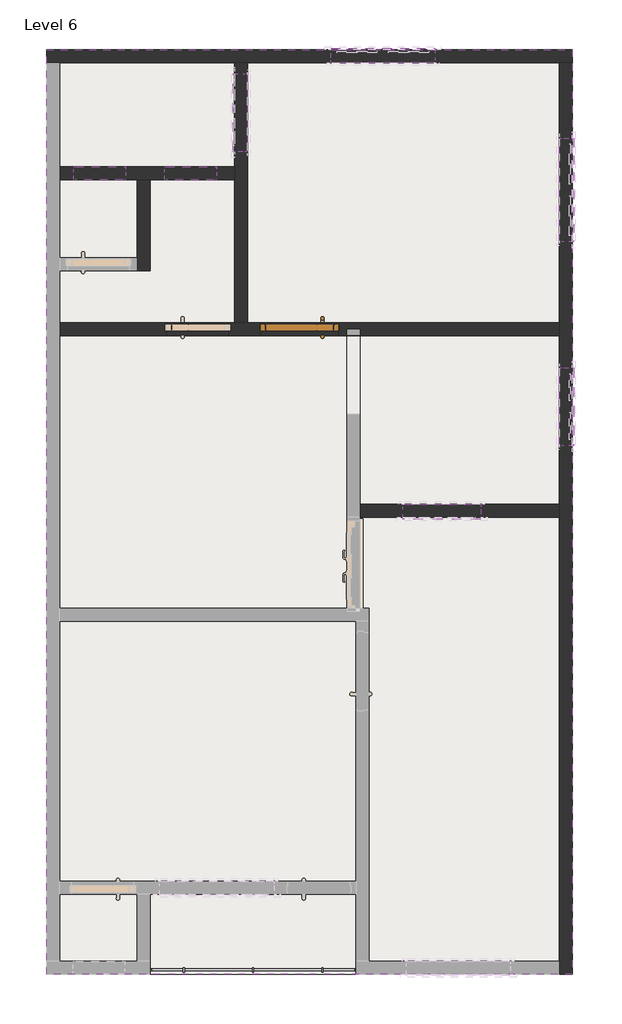
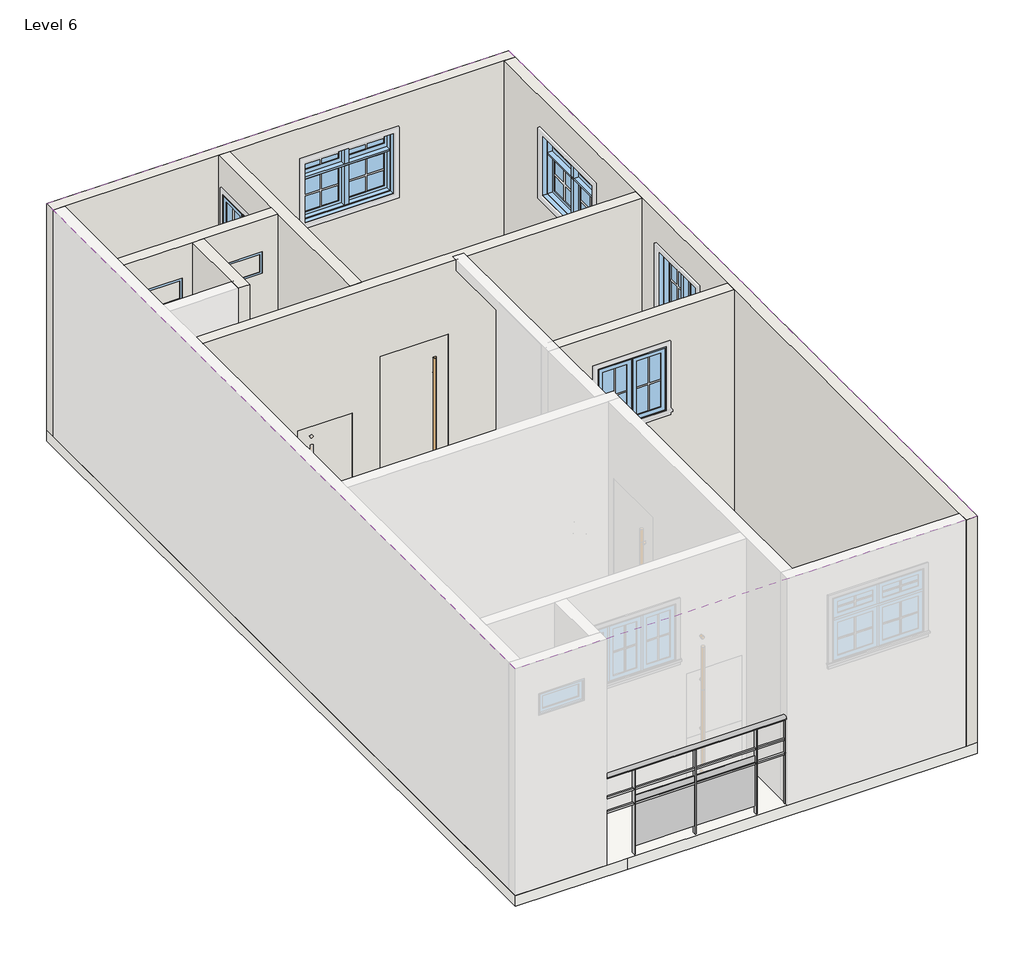
# One storey, part 2 of 3: 22 walls, 13 windows, 2 coverings, 2 railings, 1 door, 1 slab.
"""IFC4 building model written with IfcOpenShell, lengths in millimetres."""

from ifc_helpers import new_model, si_unit, point, frame, origin, place, context, project, spatial, polyline, ellipse_curve, trimmed, outline, extrude, faceted_brep, transform, mapped, element, save
from ifc_brep_helpers import plane_surface, extruded_surface, advanced_brep
from components import door_3_79df91aa, fixed_2_65c13adb, m_window_casement_double_3_e0bd8fa3, m_window_casement_double_awning_double_4_7efa9bbd

model = new_model("IFC4")

# Units and contexts
model_context = context("Model", 3, world=origin())
ifc_project = project(units=[si_unit("LENGTHUNIT", "METRE", prefix="MILLI")], contexts=[model_context])

# Site, building, storey
site = spatial("IfcSite", under=ifc_project)
building = spatial("IfcBuilding", under=site)
storey = spatial("IfcBuildingStorey", under=building, Name="Level 6", Elevation=7010.4)

# Coverings
placement = place(None, origin())
element("IfcCovering", 1, ObjectType="2' x 4' ACT System", at=placement, inside=storey, context=model_context, shape_type="SweptSolid", body=[
    extrude(outline(polyline([(-23811.2963079, -4519.7257947), (-23811.2963079, 6326.0742053), (-17639.0963079, 6326.0742053), (-17639.0963079, -4519.7257947), (-22309.2664727, -4519.7257947), (-23811.2963079, -4519.7257947)])), frame((0.0, 0.0, 10210.8), z_axis=(0.0, 0.0, 1.0), x_axis=(1.0, 0.0, 0.0)), (0.0, 0.0, 1.0), 57.15),
])
element("IfcCovering", 2, ObjectType="2' x 4' ACT System", at=placement, inside=storey, context=model_context, shape_type="SweptSolid", body=[
    extrude(outline(polyline([(-23811.2963079, -4519.7257947), (-23811.2963079, 6326.0742053), (-17639.0963079, 6326.0742053), (-17639.0963079, -4519.7257947), (-22309.2664727, -4519.7257947), (-23811.2963079, -4519.7257947)])), frame((0.0, 0.0, 10210.8), z_axis=(0.0, 0.0, 1.0), x_axis=(1.0, 0.0, 0.0)), (0.0, 0.0, 1.0), 57.15),
])

# Door
door_3_shape = door_3_79df91aa(model_context)
element("IfcDoor", 3, ObjectType="3'", at=placement, inside=storey, context=model_context, shape_type="MappedRepresentation", body=[
    mapped(door_3_shape, transform((-20839.4963079, 3049.4742053, 7010.4), x_axis=(-1.0, 0.0, 0.0), y_axis=(0.0, -1.0, 0.0), z_axis=(0.0, 0.0, 1.0))),
])

# Railings
element("IfcRailing", 4, ObjectType="Glass Panel - Bottom Fill", at=placement, inside=storey, context=model_context, shape_type="SolidModel", body=[
    advanced_brep(
    [(-22592.0963079, -4430.8257947, 8229.6), (-22592.0963079, -4507.0257947, 8229.6), (-20179.0963079, -4430.8257947, 8229.6), (-20179.0963079, -4507.0257947, 8229.6)],
    [
        (0, 1, ellipse_curve(frame((-22592.0963079, -4468.9257947, 8229.6), z_axis=(-1.0, 0.0, 0.0), x_axis=(0.0, -1.0, 0.0)), 38.1, 28.575)),
        (1, 0, ellipse_curve(frame((-22592.0963079, -4468.9257947, 8229.6), z_axis=(-1.0, 0.0, 0.0), x_axis=(0.0, -1.0, 0.0)), 38.1, 28.575)),
        (2, 3, ellipse_curve(frame((-20179.0963079, -4468.9257947, 8229.6), z_axis=(1.0, 0.0, 0.0), x_axis=(0.0, -1.0, 0.0)), 38.1, 28.575)),
        (3, 2, ellipse_curve(frame((-20179.0963079, -4468.9257947, 8229.6), z_axis=(1.0, 0.0, 0.0), x_axis=(0.0, -1.0, 0.0)), 38.1, 28.575)),
        (0, 2),
        (3, 1),
    ],
    [
        plane_surface(frame((-22592.0963079, -4468.9257947, 8229.6), z_axis=(-1.0, 0.0, 0.0), x_axis=(0.0, 1.0, 0.0))),
        plane_surface(frame((-20179.0963079, -4468.9257947, 8229.6), z_axis=(1.0, 0.0, 0.0), x_axis=(0.0, 1.0, 0.0))),
        extruded_surface(trimmed(ellipse_curve(frame((-20179.0963079, -4468.9257947, 8229.6), z_axis=(-1.0, 0.0, 0.0), x_axis=(0.0, -1.0, 0.0)), 38.1, 28.575), [point((-20179.0963079, -4430.8257947, 8229.6))], [point((-20179.0963079, -4507.0257947, 8229.6))], True, "CARTESIAN"), (-2413.0, 0.0, 0.0), 2413.0),
        extruded_surface(trimmed(ellipse_curve(frame((-20179.0963079, -4468.9257947, 8229.6), z_axis=(-1.0, 0.0, 0.0), x_axis=(0.0, -1.0, 0.0)), 38.1, 28.575), [point((-20179.0963079, -4507.0257947, 8229.6))], [point((-20179.0963079, -4430.8257947, 8229.6))], True, "CARTESIAN"), (-2413.0, 0.0, 0.0), 2413.0),
    ],
    [
        (0, [[1, 2]]),
        (1, [[3, 4]]),
        (2, [[-1, 5, -4, 6]]),
        (3, [[-2, -6, -3, -5]]),
    ],
),
    extrude(outline(polyline([(-22592.0963079, -4481.6257947), (-22592.0963079, -4456.2257947), (-20179.0963079, -4456.2257947), (-20179.0963079, -4481.6257947), (-22592.0963079, -4481.6257947)])), frame((0.0, 0.0, 7912.1), z_axis=(0.0, 0.0, 1.0), x_axis=(1.0, 0.0, 0.0)), (0.0, 0.0, 1.0), 25.4),
    extrude(outline(polyline([(-22592.0963079, -4481.6257947), (-22592.0963079, -4456.2257947), (-20179.0963079, -4456.2257947), (-20179.0963079, -4481.6257947), (-22592.0963079, -4481.6257947)])), frame((0.0, 0.0, 7708.9), z_axis=(0.0, 0.0, 1.0), x_axis=(1.0, 0.0, 0.0)), (0.0, 0.0, 1.0), 25.4),
    extrude(outline(polyline([(-20579.1463079, -4494.3257947), (-20579.1463079, -4443.5257947), (-20566.4463079, -4443.5257947), (-20566.4463079, -4494.3257947), (-20579.1463079, -4494.3257947)])), frame((0.0, 0.0, 7010.4), z_axis=(0.0, 0.0, 1.0), x_axis=(1.0, 0.0, 0.0)), (0.0, 0.0, 1.0), 1190.625),
    extrude(outline(polyline([(-21385.5963079, -4462.3906377), (-20572.7963079, -4462.3906377), (-20572.7963079, -4468.7406377), (-21385.5963079, -4468.7406377), (-21385.5963079, -4462.3906377)])), frame((0.0, 0.0, 7112.0), z_axis=(0.0, 0.0, 1.0), x_axis=(1.0, 0.0, 0.0)), (0.0, 0.0, 1.0), 711.2),
    extrude(outline(polyline([(-21391.9463079, -4494.3257947), (-21391.9463079, -4443.5257947), (-21379.2463079, -4443.5257947), (-21379.2463079, -4494.3257947), (-21391.9463079, -4494.3257947)])), frame((0.0, 0.0, 7010.4), z_axis=(0.0, 0.0, 1.0), x_axis=(1.0, 0.0, 0.0)), (0.0, 0.0, 1.0), 1190.625),
    extrude(outline(polyline([(-22198.3963079, -4462.3906377), (-21385.5963079, -4462.3906377), (-21385.5963079, -4468.7406377), (-22198.3963079, -4468.7406377), (-22198.3963079, -4462.3906377)])), frame((0.0, 0.0, 7112.0), z_axis=(0.0, 0.0, 1.0), x_axis=(1.0, 0.0, 0.0)), (0.0, 0.0, 1.0), 711.2),
    extrude(outline(polyline([(-22204.7463079, -4494.3257947), (-22204.7463079, -4443.5257947), (-22192.0463079, -4443.5257947), (-22192.0463079, -4494.3257947), (-22204.7463079, -4494.3257947)])), frame((0.0, 0.0, 7010.4), z_axis=(0.0, 0.0, 1.0), x_axis=(1.0, 0.0, 0.0)), (0.0, 0.0, 1.0), 1190.625),
    extrude(outline(polyline([(-20191.7963079, -4478.4507947), (-20191.7963079, -4459.4007947), (-20172.7463079, -4459.4007947), (-20172.7463079, -4478.4507947), (-20191.7963079, -4478.4507947)])), frame((0.0, 0.0, 7010.4), z_axis=(0.0, 0.0, 1.0), x_axis=(1.0, 0.0, 0.0)), (0.0, 0.0, 1.0), 1190.625),
    extrude(outline(polyline([(-22598.4463079, -4478.4507947), (-22598.4463079, -4459.4007947), (-22579.3963079, -4459.4007947), (-22579.3963079, -4478.4507947), (-22598.4463079, -4478.4507947)])), frame((0.0, 0.0, 7010.4), z_axis=(0.0, 0.0, 1.0), x_axis=(1.0, 0.0, 0.0)), (0.0, 0.0, 1.0), 1190.625),
])
element("IfcRailing", 5, ObjectType="Glass Panel - Bottom Fill", at=placement, inside=storey, context=model_context, shape_type="SolidModel", body=[
    advanced_brep(
    [(-22592.0963079, -4430.8257947, 8229.6), (-22592.0963079, -4507.0257947, 8229.6), (-20179.0963079, -4430.8257947, 8229.6), (-20179.0963079, -4507.0257947, 8229.6)],
    [
        (0, 1, ellipse_curve(frame((-22592.0963079, -4468.9257947, 8229.6), z_axis=(-1.0, 0.0, 0.0), x_axis=(0.0, -1.0, 0.0)), 38.1, 28.575)),
        (1, 0, ellipse_curve(frame((-22592.0963079, -4468.9257947, 8229.6), z_axis=(-1.0, 0.0, 0.0), x_axis=(0.0, -1.0, 0.0)), 38.1, 28.575)),
        (2, 3, ellipse_curve(frame((-20179.0963079, -4468.9257947, 8229.6), z_axis=(1.0, 0.0, 0.0), x_axis=(0.0, -1.0, 0.0)), 38.1, 28.575)),
        (3, 2, ellipse_curve(frame((-20179.0963079, -4468.9257947, 8229.6), z_axis=(1.0, 0.0, 0.0), x_axis=(0.0, -1.0, 0.0)), 38.1, 28.575)),
        (0, 2),
        (3, 1),
    ],
    [
        plane_surface(frame((-22592.0963079, -4468.9257947, 8229.6), z_axis=(-1.0, 0.0, 0.0), x_axis=(0.0, 1.0, 0.0))),
        plane_surface(frame((-20179.0963079, -4468.9257947, 8229.6), z_axis=(1.0, 0.0, 0.0), x_axis=(0.0, 1.0, 0.0))),
        extruded_surface(trimmed(ellipse_curve(frame((-20179.0963079, -4468.9257947, 8229.6), z_axis=(-1.0, 0.0, 0.0), x_axis=(0.0, -1.0, 0.0)), 38.1, 28.575), [point((-20179.0963079, -4430.8257947, 8229.6))], [point((-20179.0963079, -4507.0257947, 8229.6))], True, "CARTESIAN"), (-2413.0, 0.0, 0.0), 2413.0),
        extruded_surface(trimmed(ellipse_curve(frame((-20179.0963079, -4468.9257947, 8229.6), z_axis=(-1.0, 0.0, 0.0), x_axis=(0.0, -1.0, 0.0)), 38.1, 28.575), [point((-20179.0963079, -4507.0257947, 8229.6))], [point((-20179.0963079, -4430.8257947, 8229.6))], True, "CARTESIAN"), (-2413.0, 0.0, 0.0), 2413.0),
    ],
    [
        (0, [[1, 2]]),
        (1, [[3, 4]]),
        (2, [[-1, 5, -4, 6]]),
        (3, [[-2, -6, -3, -5]]),
    ],
),
    extrude(outline(polyline([(-22592.0963079, -4481.6257947), (-22592.0963079, -4456.2257947), (-20179.0963079, -4456.2257947), (-20179.0963079, -4481.6257947), (-22592.0963079, -4481.6257947)])), frame((0.0, 0.0, 7912.1), z_axis=(0.0, 0.0, 1.0), x_axis=(1.0, 0.0, 0.0)), (0.0, 0.0, 1.0), 25.4),
    extrude(outline(polyline([(-22592.0963079, -4481.6257947), (-22592.0963079, -4456.2257947), (-20179.0963079, -4456.2257947), (-20179.0963079, -4481.6257947), (-22592.0963079, -4481.6257947)])), frame((0.0, 0.0, 7708.9), z_axis=(0.0, 0.0, 1.0), x_axis=(1.0, 0.0, 0.0)), (0.0, 0.0, 1.0), 25.4),
    extrude(outline(polyline([(-20579.1463079, -4494.3257947), (-20579.1463079, -4443.5257947), (-20566.4463079, -4443.5257947), (-20566.4463079, -4494.3257947), (-20579.1463079, -4494.3257947)])), frame((0.0, 0.0, 7010.4), z_axis=(0.0, 0.0, 1.0), x_axis=(1.0, 0.0, 0.0)), (0.0, 0.0, 1.0), 1190.625),
    extrude(outline(polyline([(-21385.5963079, -4462.3906377), (-20572.7963079, -4462.3906377), (-20572.7963079, -4468.7406377), (-21385.5963079, -4468.7406377), (-21385.5963079, -4462.3906377)])), frame((0.0, 0.0, 7112.0), z_axis=(0.0, 0.0, 1.0), x_axis=(1.0, 0.0, 0.0)), (0.0, 0.0, 1.0), 711.2),
    extrude(outline(polyline([(-21391.9463079, -4494.3257947), (-21391.9463079, -4443.5257947), (-21379.2463079, -4443.5257947), (-21379.2463079, -4494.3257947), (-21391.9463079, -4494.3257947)])), frame((0.0, 0.0, 7010.4), z_axis=(0.0, 0.0, 1.0), x_axis=(1.0, 0.0, 0.0)), (0.0, 0.0, 1.0), 1190.625),
    extrude(outline(polyline([(-22198.3963079, -4462.3906377), (-21385.5963079, -4462.3906377), (-21385.5963079, -4468.7406377), (-22198.3963079, -4468.7406377), (-22198.3963079, -4462.3906377)])), frame((0.0, 0.0, 7112.0), z_axis=(0.0, 0.0, 1.0), x_axis=(1.0, 0.0, 0.0)), (0.0, 0.0, 1.0), 711.2),
    extrude(outline(polyline([(-22204.7463079, -4494.3257947), (-22204.7463079, -4443.5257947), (-22192.0463079, -4443.5257947), (-22192.0463079, -4494.3257947), (-22204.7463079, -4494.3257947)])), frame((0.0, 0.0, 7010.4), z_axis=(0.0, 0.0, 1.0), x_axis=(1.0, 0.0, 0.0)), (0.0, 0.0, 1.0), 1190.625),
    extrude(outline(polyline([(-20191.7963079, -4478.4507947), (-20191.7963079, -4459.4007947), (-20172.7463079, -4459.4007947), (-20172.7463079, -4478.4507947), (-20191.7963079, -4478.4507947)])), frame((0.0, 0.0, 7010.4), z_axis=(0.0, 0.0, 1.0), x_axis=(1.0, 0.0, 0.0)), (0.0, 0.0, 1.0), 1190.625),
    extrude(outline(polyline([(-22598.4463079, -4478.4507947), (-22598.4463079, -4459.4007947), (-22579.3963079, -4459.4007947), (-22579.3963079, -4478.4507947), (-22598.4463079, -4478.4507947)])), frame((0.0, 0.0, 7010.4), z_axis=(0.0, 0.0, 1.0), x_axis=(1.0, 0.0, 0.0)), (0.0, 0.0, 1.0), 1190.625),
])

# Slab
element("IfcSlab", 6, ObjectType="Generic - 6\"", at=placement, inside=storey, context=model_context, shape_type="SweptSolid", body=[
    extrude(outline(polyline([(-23811.2963079, 6326.0742053), (-17639.0963079, 6326.0742053), (-17639.0963079, -4519.7257947), (-22307.9023601, -4519.7257947), (-23811.2963079, -4519.7257947), (-23811.2963079, 6326.0742053)])), frame((0.0, 0.0, 6858.0), z_axis=(0.0, 0.0, 1.0), x_axis=(1.0, 0.0, 0.0)), (0.0, 0.0, 1.0), 152.4),
])

# Walls
element("IfcWall", 7, ObjectType="Generic - 6\"", at=placement, inside=storey, context=model_context, shape_type="Brep", body=[
    faceted_brep([(-23811.2963079, 6173.6742053, 7010.4), (-23658.8963079, 6173.6742053, 7010.4), (-21601.4963079, 6173.6742053, 7010.4), (-21449.0963079, 6173.6742053, 7010.4), (-17791.4963079, 6173.6742053, 7010.4), (-17639.0963079, 6173.6742053, 7010.4), (-17639.0963079, 6173.6742053, 10210.8), (-17791.4963079, 6173.6742053, 10210.8), (-21449.0963079, 6173.6742053, 10210.8), (-21601.4963079, 6173.6742053, 10210.8), (-23658.8963079, 6173.6742053, 10210.8), (-23811.2963079, 6173.6742053, 10210.8), (-19251.9963079, 6173.6742053, 9739.2), (-19251.9963079, 6173.6742053, 8839.2), (-20471.1963079, 6173.6742053, 8839.2), (-20471.1963079, 6173.6742053, 9739.2), (-23811.2963079, 6326.0742053, 7010.4), (-23811.2963079, 6326.0742053, 10210.8), (-17639.0963079, 6326.0742053, 10210.8), (-17639.0963079, 6326.0742053, 7010.4), (-19251.9963079, 6326.0742053, 9739.2), (-20471.1963079, 6326.0742053, 9739.2), (-20471.1963079, 6326.0742053, 8839.2), (-19251.9963079, 6326.0742053, 8839.2)], [[[0, 1, 2, 3, 4, 5, 6, 7, 8, 9, 10, 11], [12, 13, 14, 15]], [[16, 17, 18, 19], [20, 21, 22, 23]], [[5, 4, 3, 2, 1, 0, 16, 19]], [[11, 10, 9, 8, 7, 6, 18, 17]], [[6, 5, 19, 18]], [[0, 11, 17, 16]], [[13, 12, 20, 23]], [[14, 13, 23, 22]], [[15, 14, 22, 21]], [[12, 15, 21, 20]]]),
])
element("IfcWall", 8, ObjectType="Generic - 6\"", at=placement, inside=storey, context=model_context, shape_type="Brep", body=[
    faceted_brep([(-17791.4963079, 6173.6742053, 7010.4), (-17791.4963079, 3125.6742053, 7010.4), (-17791.4963079, 2973.2742053, 7010.4), (-17791.4963079, 992.0742053, 7010.4), (-17791.4963079, 839.6742053, 7010.4), (-17791.4963079, -4367.3257947, 7010.4), (-17791.4963079, -4519.7257947, 7010.4), (-17791.4963079, -4519.7257947, 10210.8), (-17791.4963079, -4367.3257947, 10210.8), (-17791.4963079, 839.6742053, 10210.8), (-17791.4963079, 992.0742053, 10210.8), (-17791.4963079, 2973.2742053, 10210.8), (-17791.4963079, 3125.6742053, 10210.8), (-17791.4963079, 6173.6742053, 10210.8), (-17791.4963079, 4071.8242053, 9739.2), (-17791.4963079, 4071.8242053, 8839.2), (-17791.4963079, 5291.0242053, 8839.2), (-17791.4963079, 5291.0242053, 9739.2), (-17791.4963079, 1682.6367053, 9739.2), (-17791.4963079, 1682.6367053, 8839.2), (-17791.4963079, 2597.0367053, 8839.2), (-17791.4963079, 2597.0367053, 9739.2), (-17639.0963079, 6173.6742053, 7010.4), (-17639.0963079, 6173.6742053, 10210.8), (-17639.0963079, -4519.7257947, 10210.8), (-17639.0963079, -4519.7257947, 7010.4), (-17639.0963079, 4071.8242053, 9739.2), (-17639.0963079, 5291.0242053, 9739.2), (-17639.0963079, 5291.0242053, 8839.2), (-17639.0963079, 4071.8242053, 8839.2), (-17639.0963079, 1682.6367053, 9739.2), (-17639.0963079, 2597.0367053, 9739.2), (-17639.0963079, 2597.0367053, 8839.2), (-17639.0963079, 1682.6367053, 8839.2)], [[[0, 1, 2, 3, 4, 5, 6, 7, 8, 9, 10, 11, 12, 13], [14, 15, 16, 17], [18, 19, 20, 21]], [[22, 23, 24, 25], [26, 27, 28, 29], [30, 31, 32, 33]], [[6, 5, 4, 3, 2, 1, 0, 22, 25]], [[13, 12, 11, 10, 9, 8, 7, 24, 23]], [[0, 13, 23, 22]], [[7, 6, 25, 24]], [[15, 14, 26, 29]], [[16, 15, 29, 28]], [[17, 16, 28, 27]], [[14, 17, 27, 26]], [[19, 18, 30, 33]], [[20, 19, 33, 32]], [[21, 20, 32, 31]], [[18, 21, 31, 30]]]),
])
element("IfcWall", 9, ObjectType="Generic - 6\"", at=placement, inside=storey, context=model_context, shape_type="Brep", body=[
    faceted_brep([(-21601.4963079, 6173.6742053, 7010.4), (-21601.4963079, 4954.4742053, 7010.4), (-21601.4963079, 4802.0742053, 7010.4), (-21601.4963079, 3125.6742053, 7010.4), (-21601.4963079, 3125.6742053, 10210.8), (-21601.4963079, 4802.0742053, 10210.8), (-21601.4963079, 4954.4742053, 10210.8), (-21601.4963079, 6173.6742053, 10210.8), (-21601.4963079, 6046.6742053, 9739.2), (-21601.4963079, 5132.2742053, 9739.2), (-21601.4963079, 5132.2742053, 8839.2), (-21601.4963079, 6046.6742053, 8839.2), (-21449.0963079, 6173.6742053, 7010.4), (-21449.0963079, 6173.6742053, 10210.8), (-21449.0963079, 3125.6742053, 10210.8), (-21449.0963079, 3125.6742053, 7010.4), (-21449.0963079, 6046.6742053, 9739.2), (-21449.0963079, 6046.6742053, 8839.2), (-21449.0963079, 5132.2742053, 8839.2), (-21449.0963079, 5132.2742053, 9739.2)], [[[0, 1, 2, 3, 4, 5, 6, 7], [8, 9, 10, 11]], [[12, 13, 14, 15], [16, 17, 18, 19]], [[3, 2, 1, 0, 12, 15]], [[7, 6, 5, 4, 14, 13]], [[0, 7, 13, 12]], [[4, 3, 15, 14]], [[17, 16, 8, 11]], [[18, 17, 11, 10]], [[19, 18, 10, 9]], [[16, 19, 9, 8]]]),
])
element("IfcWall", 10, ObjectType="Generic - 6\"", at=placement, inside=storey, context=model_context, shape_type="Brep", body=[
    faceted_brep([(-17791.4963079, 2973.2742053, 10210.8), (-23658.8963079, 2973.2742053, 10210.8), (-23658.8963079, 2973.2742053, 7010.4), (-22401.5963079, 2973.2742053, 7010.4), (-22401.5963079, 2973.2742053, 8534.4), (-21664.9963079, 2973.2742053, 8534.4), (-21664.9963079, 2973.2742053, 7010.4), (-21296.6963079, 2973.2742053, 7010.4), (-21296.6963079, 2973.2742053, 9199.9), (-20382.2963079, 2973.2742053, 9199.9), (-20382.2963079, 2973.2742053, 7010.4), (-17791.4963079, 2973.2742053, 7010.4), (-23658.8963079, 3125.6742053, 10210.8), (-21601.4963079, 3125.6742053, 10210.8), (-21449.0963079, 3125.6742053, 10210.8), (-17791.4963079, 3125.6742053, 10210.8), (-17791.4963079, 3125.6742053, 7010.4), (-20382.2963079, 3125.6742053, 7010.4), (-20382.2963079, 3125.6742053, 9199.9), (-21296.6963079, 3125.6742053, 9199.9), (-21296.6963079, 3125.6742053, 7010.4), (-21449.0963079, 3125.6742053, 7010.4), (-21601.4963079, 3125.6742053, 7010.4), (-21664.9963079, 3125.6742053, 7010.4), (-21664.9963079, 3125.6742053, 8534.4), (-22401.5963079, 3125.6742053, 8534.4), (-22401.5963079, 3125.6742053, 7010.4), (-23658.8963079, 3125.6742053, 7010.4), (-22401.5963079, 3105.6742053, 7010.4), (-22416.5963079, 3105.6742053, 7010.4), (-22416.5963079, 3028.6742053, 7010.4), (-22401.5963079, 3028.6742053, 7010.4), (-20382.2963079, 3028.6742053, 7010.4), (-20367.2963079, 3028.6742053, 7010.4), (-20367.2963079, 3105.6742053, 7010.4), (-20382.2963079, 3105.6742053, 7010.4), (-21296.6963079, 3028.6742053, 7010.4), (-21664.9963079, 3028.6742053, 7010.4), (-21649.9963079, 3028.6742053, 7010.4), (-21649.9963079, 3105.6742053, 7010.4), (-21664.9963079, 3105.6742053, 7010.4), (-21296.6963079, 3105.6742053, 7010.4), (-21311.6963079, 3105.6742053, 7010.4), (-21311.6963079, 3028.6742053, 7010.4), (-21296.6963079, 3105.6742053, 9199.9), (-20382.2963079, 3105.6742053, 9199.9), (-20382.2963079, 3028.6742053, 9199.9), (-21296.6963079, 3028.6742053, 9199.9), (-21311.6963079, 3105.6742053, 9214.9), (-20367.2963079, 3105.6742053, 9214.9), (-20367.2963079, 3028.6742053, 9214.9), (-21311.6963079, 3028.6742053, 9214.9), (-21664.9963079, 3105.6742053, 8534.4), (-22401.5963079, 3105.6742053, 8534.4), (-22401.5963079, 3028.6742053, 8534.4), (-21664.9963079, 3028.6742053, 8534.4), (-22416.5963079, 3105.6742053, 8549.4), (-21649.9963079, 3105.6742053, 8549.4), (-21649.9963079, 3028.6742053, 8549.4), (-22416.5963079, 3028.6742053, 8549.4)], [[[0, 1, 2, 3, 4, 5, 6, 7, 8, 9, 10, 11]], [[12, 13, 14, 15, 16, 17, 18, 19, 20, 21, 22, 23, 24, 25, 26, 27]], [[2, 27, 26, 28, 29, 30, 31, 3]], [[16, 11, 10, 32, 33, 34, 35, 17]], [[36, 7, 6, 37, 38, 39, 40, 23, 22, 21, 20, 41, 42, 43]], [[1, 0, 15, 14, 13, 12]], [[0, 11, 16, 15]], [[2, 1, 12, 27]], [[44, 19, 18, 45]], [[46, 9, 8, 47]], [[19, 44, 41, 20]], [[47, 8, 7, 36]], [[45, 18, 17, 35]], [[9, 46, 32, 10]], [[48, 49, 50, 51]], [[48, 51, 43, 42]], [[46, 47, 36, 43, 51, 50, 33, 32]], [[50, 49, 34, 33]], [[44, 45, 35, 34, 49, 48, 42, 41]], [[24, 52, 53, 25]], [[4, 54, 55, 5]], [[52, 24, 23, 40]], [[5, 55, 37, 6]], [[25, 53, 28, 26]], [[54, 4, 3, 31]], [[56, 57, 58, 59]], [[58, 57, 39, 38]], [[55, 54, 31, 30, 59, 58, 38, 37]], [[56, 59, 30, 29]], [[53, 52, 40, 39, 57, 56, 29, 28]]]),
])
element("IfcWall", 11, ObjectType="Generic - 6\"", at=placement, inside=storey, context=model_context, shape_type="SweptSolid", body=[
    extrude(outline(polyline([(7010.4, -20128.2963079), (7010.4, -17791.4963079), (10210.8, -17791.4963079), (10210.8, -20128.2963079), (7010.4, -20128.2963079)]), holes=[polyline([(9739.2, -19624.1658391), (9739.2, -18709.7658391), (8839.2, -18709.7658391), (8839.2, -19624.1658391), (9739.2, -19624.1658391)])]), frame((0.0, 839.6742053, 0.0), z_axis=(0.0, 1.0, 0.0), x_axis=(0.0, 0.0, 1.0)), (0.0, 0.0, 1.0), 152.4),
])
element("IfcWall", 12, ObjectType="Generic - 6\"", at=placement, inside=storey, context=model_context, shape_type="Brep", body=[
    faceted_brep([(-23658.8963079, 4802.0742053, 7010.4), (-22744.4963079, 4802.0742053, 7010.4), (-22592.0963079, 4802.0742053, 7010.4), (-21601.4963079, 4802.0742053, 7010.4), (-21601.4963079, 4802.0742053, 10210.8), (-22592.0963079, 4802.0742053, 10210.8), (-22744.4963079, 4802.0742053, 10210.8), (-23658.8963079, 4802.0742053, 10210.8), (-22880.5252141, 4802.0742053, 9753.6), (-22880.5252141, 4802.0742053, 9448.8), (-23490.1252141, 4802.0742053, 9448.8), (-23490.1252141, 4802.0742053, 9753.6), (-21812.6338079, 4802.0742053, 9753.6), (-21812.6338079, 4802.0742053, 9448.8), (-22422.2338079, 4802.0742053, 9448.8), (-22422.2338079, 4802.0742053, 9753.6), (-23658.8963079, 4954.4742053, 7010.4), (-23658.8963079, 4954.4742053, 10210.8), (-21601.4963079, 4954.4742053, 10210.8), (-21601.4963079, 4954.4742053, 7010.4), (-22880.5252141, 4954.4742053, 9753.6), (-23490.1252141, 4954.4742053, 9753.6), (-23490.1252141, 4954.4742053, 9448.8), (-22880.5252141, 4954.4742053, 9448.8), (-21812.6338079, 4954.4742053, 9753.6), (-22422.2338079, 4954.4742053, 9753.6), (-22422.2338079, 4954.4742053, 9448.8), (-21812.6338079, 4954.4742053, 9448.8)], [[[0, 1, 2, 3, 4, 5, 6, 7], [8, 9, 10, 11], [12, 13, 14, 15]], [[16, 17, 18, 19], [20, 21, 22, 23], [24, 25, 26, 27]], [[3, 2, 1, 0, 16, 19]], [[7, 6, 5, 4, 18, 17]], [[0, 7, 17, 16]], [[4, 3, 19, 18]], [[9, 8, 20, 23]], [[10, 9, 23, 22]], [[11, 10, 22, 21]], [[8, 11, 21, 20]], [[13, 12, 24, 27]], [[14, 13, 27, 26]], [[15, 14, 26, 25]], [[12, 15, 25, 24]]]),
])
element("IfcWall", 13, ObjectType="Generic - 6\"", at=placement, inside=storey, context=model_context, shape_type="Brep", body=[
    faceted_brep([(-22744.4963079, 4802.0742053, 7010.4), (-22744.4963079, 3887.6742053, 7010.4), (-22744.4963079, 3735.2742053, 7010.4), (-22744.4963079, 3735.2742053, 10210.8), (-22744.4963079, 3887.6742053, 10210.8), (-22744.4963079, 4802.0742053, 10210.8), (-22592.0963079, 4802.0742053, 7010.4), (-22592.0963079, 4802.0742053, 10210.8), (-22592.0963079, 3735.2742053, 10210.8), (-22592.0963079, 3735.2742053, 7010.4)], [[[0, 1, 2, 3, 4, 5]], [[6, 7, 8, 9]], [[2, 1, 0, 6, 9]], [[5, 4, 3, 8, 7]], [[0, 5, 7, 6]], [[3, 2, 9, 8]]]),
])
element("IfcWall", 14, ObjectType="Generic - 6\"", at=placement, inside=storey, context=model_context, shape_type="Brep", body=[
    faceted_brep([(-21601.4963079, 6173.6742053, 7010.4), (-21601.4963079, 4954.4742053, 7010.4), (-21601.4963079, 4802.0742053, 7010.4), (-21601.4963079, 3125.6742053, 7010.4), (-21601.4963079, 3125.6742053, 10210.8), (-21601.4963079, 4802.0742053, 10210.8), (-21601.4963079, 4954.4742053, 10210.8), (-21601.4963079, 6173.6742053, 10210.8), (-21601.4963079, 6046.6742053, 9739.2), (-21601.4963079, 5132.2742053, 9739.2), (-21601.4963079, 5132.2742053, 8839.2), (-21601.4963079, 6046.6742053, 8839.2), (-21449.0963079, 6173.6742053, 7010.4), (-21449.0963079, 6173.6742053, 10210.8), (-21449.0963079, 3125.6742053, 10210.8), (-21449.0963079, 3125.6742053, 7010.4), (-21449.0963079, 6046.6742053, 9739.2), (-21449.0963079, 6046.6742053, 8839.2), (-21449.0963079, 5132.2742053, 8839.2), (-21449.0963079, 5132.2742053, 9739.2)], [[[0, 1, 2, 3, 4, 5, 6, 7], [8, 9, 10, 11]], [[12, 13, 14, 15], [16, 17, 18, 19]], [[3, 2, 1, 0, 12, 15]], [[7, 6, 5, 4, 14, 13]], [[4, 3, 15, 14]], [[17, 16, 8, 11]], [[18, 17, 11, 10]], [[19, 18, 10, 9]], [[16, 19, 9, 8]], [[0, 7, 13, 12]]]),
])
element("IfcWall", 15, ObjectType="Generic - 6\"", at=placement, inside=storey, context=model_context, shape_type="Brep", body=[
    faceted_brep([(-23658.8963079, 2973.2742053, 7010.4), (-17791.4963079, 2973.2742053, 7010.4), (-17791.4963079, 2973.2742053, 10210.8), (-23658.8963079, 2973.2742053, 10210.8), (-23658.8963079, 3125.6742053, 7010.4), (-23658.8963079, 3125.6742053, 10210.8), (-21601.4963079, 3125.6742053, 10210.8), (-21449.0963079, 3125.6742053, 10210.8), (-17791.4963079, 3125.6742053, 10210.8), (-17791.4963079, 3125.6742053, 7010.4), (-21449.0963079, 3125.6742053, 7010.4), (-21601.4963079, 3125.6742053, 7010.4)], [[[0, 1, 2, 3]], [[4, 5, 6, 7, 8, 9, 10, 11]], [[1, 0, 4, 11, 10, 9]], [[3, 2, 8, 7, 6, 5]], [[0, 3, 5, 4]], [[2, 1, 9, 8]]]),
])
element("IfcWall", 16, ObjectType="Generic - 6\"", at=placement, inside=storey, context=model_context, shape_type="SweptSolid", body=[
    extrude(outline(polyline([(7010.4, -20128.2963079), (7010.4, -17791.4963079), (10210.8, -17791.4963079), (10210.8, -20128.2963079), (7010.4, -20128.2963079)]), holes=[polyline([(9739.2, -19624.1658391), (9739.2, -18709.7658391), (8839.2, -18709.7658391), (8839.2, -19624.1658391), (9739.2, -19624.1658391)])]), frame((0.0, 839.6742053, 0.0), z_axis=(0.0, 1.0, 0.0), x_axis=(0.0, 0.0, 1.0)), (0.0, 0.0, 1.0), 152.4),
])
element("IfcWall", 17, ObjectType="Generic - 6\"", at=placement, inside=storey, context=model_context, shape_type="Brep", body=[
    faceted_brep([(-23658.8963079, 4802.0742053, 7010.4), (-22744.4963079, 4802.0742053, 7010.4), (-22592.0963079, 4802.0742053, 7010.4), (-21601.4963079, 4802.0742053, 7010.4), (-21601.4963079, 4802.0742053, 10210.8), (-22592.0963079, 4802.0742053, 10210.8), (-22744.4963079, 4802.0742053, 10210.8), (-23658.8963079, 4802.0742053, 10210.8), (-23658.8963079, 4954.4742053, 7010.4), (-23658.8963079, 4954.4742053, 10210.8), (-21601.4963079, 4954.4742053, 10210.8), (-21601.4963079, 4954.4742053, 7010.4)], [[[0, 1, 2, 3, 4, 5, 6, 7]], [[8, 9, 10, 11]], [[3, 2, 1, 0, 8, 11]], [[7, 6, 5, 4, 10, 9]], [[4, 3, 11, 10]], [[0, 7, 9, 8]]]),
])
element("IfcWall", 18, ObjectType="Generic - 6\"", at=placement, inside=storey, context=model_context, shape_type="SweptSolid", body=[
    extrude(outline(polyline([(-22744.4963079, 3887.6742053), (-22744.4963079, 4802.0742053), (-22592.0963079, 4802.0742053), (-22592.0963079, 3887.6742053), (-22744.4963079, 3887.6742053)])), frame((0.0, 0.0, 7010.4), z_axis=(0.0, 0.0, 1.0), x_axis=(1.0, 0.0, 0.0)), (0.0, 0.0, 1.0), 3200.4),
])
element("IfcWall", 19, ObjectType="Generic - 6\"", at=placement, inside=storey, context=model_context, shape_type="Brep", body=[
    faceted_brep([(-21601.4963079, 6173.6742053, 7010.4), (-21601.4963079, 4954.4742053, 7010.4), (-21601.4963079, 4802.0742053, 7010.4), (-21601.4963079, 3125.6742053, 7010.4), (-21601.4963079, 3125.6742053, 10210.8), (-21601.4963079, 4802.0742053, 10210.8), (-21601.4963079, 4954.4742053, 10210.8), (-21601.4963079, 6173.6742053, 10210.8), (-21601.4963079, 6046.6742053, 9739.2), (-21601.4963079, 5132.2742053, 9739.2), (-21601.4963079, 5132.2742053, 8839.2), (-21601.4963079, 6046.6742053, 8839.2), (-21449.0963079, 6173.6742053, 7010.4), (-21449.0963079, 6173.6742053, 10210.8), (-21449.0963079, 3125.6742053, 10210.8), (-21449.0963079, 3125.6742053, 7010.4), (-21449.0963079, 6046.6742053, 9739.2), (-21449.0963079, 6046.6742053, 8839.2), (-21449.0963079, 5132.2742053, 8839.2), (-21449.0963079, 5132.2742053, 9739.2)], [[[0, 1, 2, 3, 4, 5, 6, 7], [8, 9, 10, 11]], [[12, 13, 14, 15], [16, 17, 18, 19]], [[3, 2, 1, 0, 12, 15]], [[7, 6, 5, 4, 14, 13]], [[4, 3, 15, 14]], [[17, 16, 8, 11]], [[18, 17, 11, 10]], [[19, 18, 10, 9]], [[16, 19, 9, 8]], [[0, 7, 13, 12]]]),
])
element("IfcWall", 20, ObjectType="Generic - 6\"", at=placement, inside=storey, context=model_context, shape_type="Brep", body=[
    faceted_brep([(-23658.8963079, 2973.2742053, 7010.4), (-17791.4963079, 2973.2742053, 7010.4), (-17791.4963079, 2973.2742053, 10210.8), (-23658.8963079, 2973.2742053, 10210.8), (-23658.8963079, 3125.6742053, 7010.4), (-23658.8963079, 3125.6742053, 10210.8), (-21601.4963079, 3125.6742053, 10210.8), (-21449.0963079, 3125.6742053, 10210.8), (-17791.4963079, 3125.6742053, 10210.8), (-17791.4963079, 3125.6742053, 7010.4), (-21449.0963079, 3125.6742053, 7010.4), (-21601.4963079, 3125.6742053, 7010.4)], [[[0, 1, 2, 3]], [[4, 5, 6, 7, 8, 9, 10, 11]], [[1, 0, 4, 11, 10, 9]], [[3, 2, 8, 7, 6, 5]], [[0, 3, 5, 4]], [[2, 1, 9, 8]]]),
])
element("IfcWall", 21, ObjectType="Generic - 6\"", at=placement, inside=storey, context=model_context, shape_type="SweptSolid", body=[
    extrude(outline(polyline([(7010.4, -20128.2963079), (7010.4, -17791.4963079), (10210.8, -17791.4963079), (10210.8, -20128.2963079), (7010.4, -20128.2963079)]), holes=[polyline([(9739.2, -19624.1658391), (9739.2, -18709.7658391), (8839.2, -18709.7658391), (8839.2, -19624.1658391), (9739.2, -19624.1658391)])]), frame((0.0, 839.6742053, 0.0), z_axis=(0.0, 1.0, 0.0), x_axis=(0.0, 0.0, 1.0)), (0.0, 0.0, 1.0), 152.4),
])
element("IfcWall", 22, ObjectType="Generic - 6\"", at=placement, inside=storey, context=model_context, shape_type="Brep", body=[
    faceted_brep([(-23658.8963079, 4802.0742053, 7010.4), (-22744.4963079, 4802.0742053, 7010.4), (-22592.0963079, 4802.0742053, 7010.4), (-21601.4963079, 4802.0742053, 7010.4), (-21601.4963079, 4802.0742053, 10210.8), (-22592.0963079, 4802.0742053, 10210.8), (-22744.4963079, 4802.0742053, 10210.8), (-23658.8963079, 4802.0742053, 10210.8), (-23658.8963079, 4954.4742053, 7010.4), (-23658.8963079, 4954.4742053, 10210.8), (-21601.4963079, 4954.4742053, 10210.8), (-21601.4963079, 4954.4742053, 7010.4)], [[[0, 1, 2, 3, 4, 5, 6, 7]], [[8, 9, 10, 11]], [[3, 2, 1, 0, 8, 11]], [[7, 6, 5, 4, 10, 9]], [[4, 3, 11, 10]], [[0, 7, 9, 8]]]),
])
element("IfcWall", 23, ObjectType="Generic - 6\"", at=placement, inside=storey, context=model_context, shape_type="SweptSolid", body=[
    extrude(outline(polyline([(-22744.4963079, 3887.6742053), (-22744.4963079, 4802.0742053), (-22592.0963079, 4802.0742053), (-22592.0963079, 3887.6742053), (-22744.4963079, 3887.6742053)])), frame((0.0, 0.0, 7010.4), z_axis=(0.0, 0.0, 1.0), x_axis=(1.0, 0.0, 0.0)), (0.0, 0.0, 1.0), 3200.4),
])
element("IfcWall", 24, ObjectType="Generic - 6\"", at=placement, inside=storey, context=model_context, shape_type="Brep", body=[
    faceted_brep([(-21601.4963079, 6173.6742053, 7010.4), (-21601.4963079, 4954.4742053, 7010.4), (-21601.4963079, 4802.0742053, 7010.4), (-21601.4963079, 3125.6742053, 7010.4), (-21601.4963079, 3125.6742053, 10210.8), (-21601.4963079, 4802.0742053, 10210.8), (-21601.4963079, 4954.4742053, 10210.8), (-21601.4963079, 6173.6742053, 10210.8), (-21601.4963079, 6046.6742053, 9739.2), (-21601.4963079, 5132.2742053, 9739.2), (-21601.4963079, 5132.2742053, 8839.2), (-21601.4963079, 6046.6742053, 8839.2), (-21449.0963079, 6173.6742053, 7010.4), (-21449.0963079, 6173.6742053, 10210.8), (-21449.0963079, 3125.6742053, 10210.8), (-21449.0963079, 3125.6742053, 7010.4), (-21449.0963079, 6046.6742053, 9739.2), (-21449.0963079, 6046.6742053, 8839.2), (-21449.0963079, 5132.2742053, 8839.2), (-21449.0963079, 5132.2742053, 9739.2)], [[[0, 1, 2, 3, 4, 5, 6, 7], [8, 9, 10, 11]], [[12, 13, 14, 15], [16, 17, 18, 19]], [[3, 2, 1, 0, 12, 15]], [[7, 6, 5, 4, 14, 13]], [[4, 3, 15, 14]], [[17, 16, 8, 11]], [[18, 17, 11, 10]], [[19, 18, 10, 9]], [[16, 19, 9, 8]], [[0, 7, 13, 12]]]),
])
element("IfcWall", 25, ObjectType="Generic - 6\"", at=placement, inside=storey, context=model_context, shape_type="Brep", body=[
    faceted_brep([(-23658.8963079, 2973.2742053, 7010.4), (-17791.4963079, 2973.2742053, 7010.4), (-17791.4963079, 2973.2742053, 10210.8), (-23658.8963079, 2973.2742053, 10210.8), (-23658.8963079, 3125.6742053, 7010.4), (-23658.8963079, 3125.6742053, 10210.8), (-21601.4963079, 3125.6742053, 10210.8), (-21449.0963079, 3125.6742053, 10210.8), (-17791.4963079, 3125.6742053, 10210.8), (-17791.4963079, 3125.6742053, 7010.4), (-21449.0963079, 3125.6742053, 7010.4), (-21601.4963079, 3125.6742053, 7010.4)], [[[0, 1, 2, 3]], [[4, 5, 6, 7, 8, 9, 10, 11]], [[1, 0, 4, 11, 10, 9]], [[3, 2, 8, 7, 6, 5]], [[0, 3, 5, 4]], [[2, 1, 9, 8]]]),
])
element("IfcWall", 26, ObjectType="Generic - 6\"", at=placement, inside=storey, context=model_context, shape_type="SweptSolid", body=[
    extrude(outline(polyline([(7010.4, -20128.2963079), (7010.4, -17791.4963079), (10210.8, -17791.4963079), (10210.8, -20128.2963079), (7010.4, -20128.2963079)]), holes=[polyline([(9739.2, -19624.1658391), (9739.2, -18709.7658391), (8839.2, -18709.7658391), (8839.2, -19624.1658391), (9739.2, -19624.1658391)])]), frame((0.0, 839.6742053, 0.0), z_axis=(0.0, 1.0, 0.0), x_axis=(0.0, 0.0, 1.0)), (0.0, 0.0, 1.0), 152.4),
])
element("IfcWall", 27, ObjectType="Generic - 6\"", at=placement, inside=storey, context=model_context, shape_type="Brep", body=[
    faceted_brep([(-23658.8963079, 4802.0742053, 7010.4), (-22744.4963079, 4802.0742053, 7010.4), (-22592.0963079, 4802.0742053, 7010.4), (-21601.4963079, 4802.0742053, 7010.4), (-21601.4963079, 4802.0742053, 10210.8), (-22592.0963079, 4802.0742053, 10210.8), (-22744.4963079, 4802.0742053, 10210.8), (-23658.8963079, 4802.0742053, 10210.8), (-23658.8963079, 4954.4742053, 7010.4), (-23658.8963079, 4954.4742053, 10210.8), (-21601.4963079, 4954.4742053, 10210.8), (-21601.4963079, 4954.4742053, 7010.4)], [[[0, 1, 2, 3, 4, 5, 6, 7]], [[8, 9, 10, 11]], [[3, 2, 1, 0, 8, 11]], [[7, 6, 5, 4, 10, 9]], [[4, 3, 11, 10]], [[0, 7, 9, 8]]]),
])
element("IfcWall", 28, ObjectType="Generic - 6\"", at=placement, inside=storey, context=model_context, shape_type="SweptSolid", body=[
    extrude(outline(polyline([(-22744.4963079, 3887.6742053), (-22744.4963079, 4802.0742053), (-22592.0963079, 4802.0742053), (-22592.0963079, 3887.6742053), (-22744.4963079, 3887.6742053)])), frame((0.0, 0.0, 7010.4), z_axis=(0.0, 0.0, 1.0), x_axis=(1.0, 0.0, 0.0)), (0.0, 0.0, 1.0), 3200.4),
])

# Windows
fixed_2_shape = fixed_2_65c13adb(model_context)
element("IfcWindow", 29, ObjectType="Fixed : 2'", at=placement, inside=storey, context=model_context, shape_type="MappedRepresentation", body=[
    mapped(fixed_2_shape, transform((-23147.2252141, 4878.2742053, 8534.4), x_axis=(1.0, 0.0, 0.0), y_axis=(0.0, 1.0, 0.0), z_axis=(0.0, 0.0, 1.0))),
])
element("IfcWindow", 30, ObjectType="Fixed : 2'", at=placement, inside=storey, context=model_context, shape_type="MappedRepresentation", body=[
    mapped(fixed_2_shape, transform((-22079.3338079, 4878.2742053, 8534.4), x_axis=(1.0, 0.0, 0.0), y_axis=(0.0, 1.0, 0.0), z_axis=(0.0, 0.0, 1.0))),
])
m_window_casement_double_3_shape = m_window_casement_double_3_e0bd8fa3(model_context)
element("IfcWindow", 31, ObjectType="M_Window-Casement-Double : 3'", at=placement, inside=storey, context=model_context, shape_type="MappedRepresentation", body=[
    mapped(m_window_casement_double_3_shape, transform((-19166.9658391, 915.8742053, 7939.2), x_axis=(-1.0, 0.0, 0.0), y_axis=(0.0, -1.0, 0.0), z_axis=(0.0, 0.0, 1.0))),
])
element("IfcWindow", 32, ObjectType="M_Window-Casement-Double : 3'", at=placement, inside=storey, context=model_context, shape_type="MappedRepresentation", body=[
    mapped(m_window_casement_double_3_shape, transform((-17715.2963079, 2139.8367053, 7939.2), x_axis=(0.0, -1.0, 0.0), y_axis=(1.0, 0.0, 0.0), z_axis=(0.0, 0.0, 1.0))),
])
element("IfcWindow", 33, ObjectType="M_Window-Casement-Double : 3'", at=placement, inside=storey, context=model_context, shape_type="MappedRepresentation", body=[
    mapped(m_window_casement_double_3_shape, transform((-21525.2963079, 5589.4742053, 7939.2), x_axis=(0.0, 1.0, 0.0), y_axis=(-1.0, 0.0, 0.0), z_axis=(0.0, 0.0, 1.0))),
])
element("IfcWindow", 34, ObjectType="M_Window-Casement-Double : 3'", at=placement, inside=storey, context=model_context, shape_type="MappedRepresentation", body=[
    mapped(m_window_casement_double_3_shape, transform((-19166.9658391, 915.8742053, 7939.2), x_axis=(-1.0, 0.0, 0.0), y_axis=(0.0, -1.0, 0.0), z_axis=(0.0, 0.0, 1.0))),
])
element("IfcWindow", 35, ObjectType="M_Window-Casement-Double : 3'", at=placement, inside=storey, context=model_context, shape_type="MappedRepresentation", body=[
    mapped(m_window_casement_double_3_shape, transform((-21525.2963079, 5589.4742053, 7939.2), x_axis=(0.0, 1.0, 0.0), y_axis=(-1.0, 0.0, 0.0), z_axis=(0.0, 0.0, 1.0))),
])
element("IfcWindow", 36, ObjectType="M_Window-Casement-Double : 3'", at=placement, inside=storey, context=model_context, shape_type="MappedRepresentation", body=[
    mapped(m_window_casement_double_3_shape, transform((-19166.9658391, 915.8742053, 7939.2), x_axis=(-1.0, 0.0, 0.0), y_axis=(0.0, -1.0, 0.0), z_axis=(0.0, 0.0, 1.0))),
])
element("IfcWindow", 37, ObjectType="M_Window-Casement-Double : 3'", at=placement, inside=storey, context=model_context, shape_type="MappedRepresentation", body=[
    mapped(m_window_casement_double_3_shape, transform((-21525.2963079, 5589.4742053, 7939.2), x_axis=(0.0, 1.0, 0.0), y_axis=(-1.0, 0.0, 0.0), z_axis=(0.0, 0.0, 1.0))),
])
element("IfcWindow", 38, ObjectType="M_Window-Casement-Double : 3'", at=placement, inside=storey, context=model_context, shape_type="MappedRepresentation", body=[
    mapped(m_window_casement_double_3_shape, transform((-19166.9658391, 915.8742053, 7939.2), x_axis=(-1.0, 0.0, 0.0), y_axis=(0.0, -1.0, 0.0), z_axis=(0.0, 0.0, 1.0))),
])
element("IfcWindow", 39, ObjectType="M_Window-Casement-Double : 3'", at=placement, inside=storey, context=model_context, shape_type="MappedRepresentation", body=[
    mapped(m_window_casement_double_3_shape, transform((-21525.2963079, 5589.4742053, 7939.2), x_axis=(0.0, 1.0, 0.0), y_axis=(-1.0, 0.0, 0.0), z_axis=(0.0, 0.0, 1.0))),
])
m_window_casement_double_awning_double_4_shape = m_window_casement_double_awning_double_4_7efa9bbd(model_context)
element("IfcWindow", 40, ObjectType="M_Window-Casement-Double-Awning-Double : 4'", at=placement, inside=storey, context=model_context, shape_type="MappedRepresentation", body=[
    mapped(m_window_casement_double_awning_double_4_shape, transform((-19861.5963079, 6249.8742053, 7939.2), x_axis=(1.0, 0.0, 0.0), y_axis=(0.0, 1.0, 0.0), z_axis=(0.0, 0.0, 1.0))),
])
element("IfcWindow", 41, ObjectType="M_Window-Casement-Double-Awning-Double : 4'", at=placement, inside=storey, context=model_context, shape_type="MappedRepresentation", body=[
    mapped(m_window_casement_double_awning_double_4_shape, transform((-17715.2963079, 4681.4242053, 7939.2), x_axis=(0.0, -1.0, 0.0), y_axis=(1.0, 0.0, 0.0), z_axis=(0.0, 0.0, 1.0))),
])

save(model, "model.ifc")

# Revit data of these elements
# Type "2' x 4' ACT System"
#   Assembly Code = "C3030210"
#   built-in parameter 1002203 = 1 (stored number, unit not read)
#   built-in parameter 1002202 = 1 (stored number, unit not read)
#   Layers, outside or top first: 0' - 1 5/8" "Default" (function 1); 0' - 0 5/8" "Acoustic Ceiling Tile 24 x 48" (function 5)
# Type "3'"
#   Type Mark = "10"
#   Water resistance = "up to Class E900, EN 12208:2001"
#   Uniclass2015Version = "v1.21"
#   Uniclass2015Reference = "Ss_25_30_20_30"
#   Uniclass2015Description = "Frame and door leaf system"
#   URL = "www.aluprof.com"
#   Type IFC Predefined Type = "USERDEFINED"
#   Right-hand / Left-hand door [instance default] = ""
#   Resistance to wind load = "up to Class C5/B5, EN 12210:2001"
#   Insert type = "ST"
#   Hardware [instance default] = ""
#   Product page = "https://aluprof.com/en/architects/offer/window-and-door-systems/panel-doors#visualisation"
#   Operation = "SinglePanelOutwardOpening"
#   Opening type = "Outward"
#   NBSReference = "25-50-20/125"
#   NBSDescription = "Frame and door leaf system"
#   Important = "The actual acceptable construction dimensions are dependent on the selection of profiles and hardware, glazing type, construction weight and the construction’s operating conditions. These should be determined by a suitably qualified person, and using ALUPROF’s calculation software"
#   IfcExportType = "USERDEFINED"
#   IfcExportAs = "IfcDoorType"
#   Handle type [instance default] = ""
#   Manufacturer = "ALUPROF SA"
#   Export Type to IFC As = "IfcDoorType"
#   Door sill type [instance default] = ""
#   Description = "External single-leaf panel door outward opening"
#   Model = "MB-86 ST Panel Door AD07"
#   Content of the recyclate in the material = "69.2%"
#   COBie.Type.WarrantyDurationParts = ""
#   COBie.Type.Name = ""
#   COBie.Type.Manufacturer = "ALUPROF SA"
#   COBie.Space.Name = ""
#   COBie.Floor.Name = ""
#   COBie.Facility.Name = ""
#   COBie.CreatedOn = ""
#   COBie.Component.WarrantyStartDate = ""
#   COBie.Component.Name = "MB-86 ST Panel Door AD07"
#   Burglar resistance = "RC2"
#   Air permeability = "up to Class 4, EN 12207:2001"
#   Width of the active leaf = 2' - 8.17717"
#   Placement in wall = 0' - 0.7874"
#   Thickness = 0' - 3.0315"
#   Height of the opening sash = 6' - 11.64173"
#   Handle Offset = 3' - 5.33858"
#   Rough Height = 7' - 4.61024"
#   Rough Width = 3' - 1.1811"
#   Height = 7' - 2.20079"
#   Width = 3' - 0"
#   Construction depth = 0' - 3.0315"
#   Clear opening width = 2' - 3.94882"
#   Clear opening height = 6' - 10.67717"
#   Height of the array = 1' - 1.44816"
#   Schedule No. [instance default] = 1
#   Handrail [instance default] = yes
#   IsExternal = yes
#   Handle [instance default] = no
#   Door closer [instance default] = no
#   Function = 1
#   COBie.Type = yes
#   COBie = yes
#   Access control [instance default] = no
#   Panel = element 346771
#   Wall Closure = (empty or 0)
# Type "Glass Panel - Bottom Fill"
#   Assembly Code = "C2010400"
#   built-in parameter 1008612 = 0.0416667 (stored number, unit not read)
#   built-in parameter 1008611 = 0.0416667 (stored number, unit not read)
#   built-in parameter 1008609 = 0.333333 (stored number, unit not read)
#   built-in parameter 1008604 = 0.166667 (stored number, unit not read)
#   built-in parameter 1008603 = 0.166667 (stored number, unit not read)
#   Railing Height = 4' - 0"
#   built-in parameter 1008630 = 2
#   built-in parameter 1008610 = 2
#   built-in parameter 1008618 = Baluster - Square : 3/4"
# Type "Generic - 6\""
#   Assembly Code = "B1010"
#   Function = 0
#   Layers, outside or top first: 0' - 6" no material (function 1)
# Type "Generic - 6\""
#   Assembly Code = "B2010"
#   Layers, outside or top first: 0' - 6" no material (function 1)
# Type "Fixed : 2'"
#   Type Mark = "16"
#   Assembly Code = "B2020100"
#   Height = 1' - 0"
#   Default Sill Height = 3' - 0"
#   Width = 2' - 0"
#   Window Inset = 0' - 0 3/4"
#   Glass Pane Material = Glass
#   Sash Material = Sash
#   Wall Closure = (empty or 0)
# Type "M_Window-Casement-Double : 3'"
#   Type Mark = "13"
#   Fire Rating = "0.5h"
#   Assembly Code = "B2020100"
#   Analytic Construction = "Double glazing - domestic"
#   Frame Extension [instance default] = 0' - 0 1/4"
#   Window Inset [instance default] = 0' - 0"
#   Wall Thickness [instance default] = 0' - 5.90551"
#   Interior Wall Closure [instance default] = 0' - 2.15551"
#   Half Width = 1' - 6"
#   Visual Light Transmittance = 0.81
#   Thermal Resistance (R) = 1.8146 (h·ft²·°F)/BTU
#   Solar Heat Gain Coefficient = 0.76
#   Rough Width = 3' - 0.59055"
#   Rough Height = 3' - 0.02362"
#   Height = 2' - 11.43307"
#   Heat Transfer Coefficient (U) = 0.5511 BTU/(h·ft²·°F)
#   Exterior Wall Closure [instance default] = 0' - 1.25197"
#   Extension Jamb [instance default] = 0' - 2.15551"
#   Default Sill Height = 2' - 11.43307"
#   Width = 3' - 0"
#   Muntin Visibility = yes
#   Interior Trim Visibility [instance default] = yes
#   Exterior Trim Visibility [instance default] = yes
#   Extension Jamb Visibility [instance default] = yes
#   Interior Trim Material = Wood - Stained
#   Muntin Pattern = M_Muntin Pattern_2x2 : M_Muntin Pattern_2x2
#   Interior Trim = M_Trim-Window-Interior-Flat : Picture Frame
#   Interior Frame Material = Wood - Stained
#   Glass Panel Material = Glass
#   Exterior Trim Material = Clad - White
#   Exterior Trim = M_Trim-Window-Exterior-Flat : with Sill
#   Exterior Frame Material = Clad - White
#   Wall Closure = (empty or 0)
# Type "M_Window-Casement-Double-Awning-Double : 4'"
#   Type Mark = "11"
#   Fire Rating = "0.5h"
#   Assembly Code = "B2020100"
#   Analytic Construction = "Double glazing - domestic"
#   Window Inset [instance default] = 0' - 0"
#   Wall Thickness [instance default] = 0' - 5.90551"
#   Interior Wall Closure [instance default] = 0' - 2.15551"
#   Half Width = 2' - 0"
#   Visual Light Transmittance = 0.81
#   Transom Height = 0' - 11.81102"
#   Thermal Resistance (R) = 1.8146 (h·ft²·°F)/BTU
#   Solar Heat Gain Coefficient = 0.76
#   Rough Width = 4' - 0.59055"
#   Rough Height = 3' - 0.02362"
#   Open Window Height = 1' - 11.62205"
#   Frame Extension [instance default] = 0' - 0 1/4"
#   Height = 2' - 11.43307"
#   Heat Transfer Coefficient (U) = 0.5511 BTU/(h·ft²·°F)
#   Exterior Wall Closure [instance default] = 0' - 1.25197"
#   Extension Jamb [instance default] = 0' - 2.15551"
#   Default Sill Height = 2' - 11.43307"
#   Width = 4' - 0"
#   Top Muntin Visibility = yes
#   Bottom Muntin Visibility = yes
#   Interior Trim Visibility [instance default] = yes
#   Exterior Trim Visibility [instance default] = yes
#   Extension Jamb Visibility [instance default] = yes
#   Interior Trim Material = Wood - Stained
#   Muntin Pattern = M_Muntin Pattern_2x2 : M_Muntin Pattern_2x2
#   Interior Trim = M_Trim-Window-Interior-Flat : Picture Frame
#   Interior Frame Material = Wood - Stained
#   Glass Panel Material = Glass
#   Exterior Trim Material = Clad - White
#   Exterior Trim = M_Trim-Window-Exterior-Flat : with Sill
#   Exterior Frame Material = Clad - White
#   Wall Closure = (empty or 0)
# Elements 1, 2 (IfcCovering, "2' x 4' ACT System")
#   Height Offset From Level = 10' - 6"
#   Phase Created = New Construction
#   Materials on its faces: "Acoustic Ceiling Tile 24 x 48", "Default"
# Element 3 (IfcDoor, "3'")
#   Right-hand / Left-hand door = ""
#   Hardware = ""
#   Handle type = ""
#   Door sill type = ""
#   Schedule No. = 1
#   Handrail = yes
#   Handle = no
#   Door closer = no
#   Access control = no
#   Phase Created = New Construction
# Elements 4, 5 (IfcRailing, "Glass Panel - Bottom Fill")
#   Phase Created = New Construction
#   Materials on its faces: "Glass"
# Element 6 (IfcSlab, "Generic - 6\"")
#   built-in parameter 1001955 = 3.14159 (stored number, unit not read)
#   Height Offset From Level = 0' - 0"
#   Phase Created = New Construction
#   Materials on its faces: "Parking Stripe", "Default Floor"
# Elements 7, 8 (IfcWall, "Generic - 6\"")
#   Top Offset = 0' - 0"
#   Base Offset = 0' - 0"
#   Unconnected Height = 10' - 6"
#   wall height = 10' - 6"
#   Phase Created = New Construction
#   Base Constraint = Level 6
#   Materials on its faces: "Default Wall", "Parking Stripe"
# Elements 9, 10, 11, 12, 13, 14, 15, 16, 17, 18, 19, 20, 21, 22, 23, 24, 25, 26, 27, 28 (IfcWall, "Generic - 6\"")
#   Top Offset = 0' - 0"
#   Base Offset = 0' - 0"
#   Unconnected Height = 10' - 6"
#   wall height = 10' - 6"
#   Phase Created = New Construction
#   Base Constraint = Level 6
#   Materials on its faces: "Default Wall"
# Element 29 (IfcWindow, "Fixed : 2'")
#   Mark = "29"
#   Phase Created = New Construction
#   Materials on its faces: "Sash", "Glass"
# Element 30 (IfcWindow, "Fixed : 2'")
#   Mark = "30"
#   Phase Created = New Construction
#   Materials on its faces: "Sash", "Glass"
# Element 31 (IfcWindow, "M_Window-Casement-Double : 3'")
#   Mark = "24"
#   Window Inset = 0' - 0"
#   Interior Wall Closure = 0' - 2.15551"
#   Frame Extension = 0' - 0 1/4"
#   Exterior Wall Closure = 0' - 1.25197"
#   Interior Trim Visibility = yes
#   Exterior Trim Visibility = yes
#   Phase Created = New Construction
#   Materials on its faces: "Wood - Stained", "Glass", "Clad - White"
# Element 32 (IfcWindow, "M_Window-Casement-Double : 3'")
#   Mark = "25"
#   Window Inset = 0' - 0"
#   Interior Wall Closure = 0' - 2.15551"
#   Frame Extension = 0' - 0 1/4"
#   Exterior Wall Closure = 0' - 1.25197"
#   Interior Trim Visibility = yes
#   Exterior Trim Visibility = yes
#   Phase Created = New Construction
#   Materials on its faces: "Wood - Stained", "Glass", "Clad - White"
# Element 33 (IfcWindow, "M_Window-Casement-Double : 3'")
#   Mark = "26"
#   Window Inset = 0' - 0"
#   Interior Wall Closure = 0' - 2.15551"
#   Frame Extension = 0' - 0 1/4"
#   Exterior Wall Closure = 0' - 1.25197"
#   Interior Trim Visibility = yes
#   Exterior Trim Visibility = yes
#   Phase Created = New Construction
#   Materials on its faces: "Wood - Stained", "Glass", "Clad - White"
# Element 34 (IfcWindow, "M_Window-Casement-Double : 3'")
#   Mark = "64"
#   Window Inset = 0' - 0"
#   Interior Wall Closure = 0' - 2.15551"
#   Frame Extension = 0' - 0 1/4"
#   Exterior Wall Closure = 0' - 1.25197"
#   Interior Trim Visibility = yes
#   Exterior Trim Visibility = yes
#   Phase Created = New Construction
#   Materials on its faces: "Wood - Stained", "Glass", "Clad - White"
# Element 35 (IfcWindow, "M_Window-Casement-Double : 3'")
#   Mark = "66"
#   Window Inset = 0' - 0"
#   Interior Wall Closure = 0' - 2.15551"
#   Frame Extension = 0' - 0 1/4"
#   Exterior Wall Closure = 0' - 1.25197"
#   Interior Trim Visibility = yes
#   Exterior Trim Visibility = yes
#   Phase Created = New Construction
#   Materials on its faces: "Wood - Stained", "Glass", "Clad - White"
# Element 36 (IfcWindow, "M_Window-Casement-Double : 3'")
#   Mark = "94"
#   Window Inset = 0' - 0"
#   Interior Wall Closure = 0' - 2.15551"
#   Frame Extension = 0' - 0 1/4"
#   Exterior Wall Closure = 0' - 1.25197"
#   Interior Trim Visibility = yes
#   Exterior Trim Visibility = yes
#   Phase Created = New Construction
#   Materials on its faces: "Wood - Stained", "Glass", "Clad - White"
# Element 37 (IfcWindow, "M_Window-Casement-Double : 3'")
#   Mark = "96"
#   Window Inset = 0' - 0"
#   Interior Wall Closure = 0' - 2.15551"
#   Frame Extension = 0' - 0 1/4"
#   Exterior Wall Closure = 0' - 1.25197"
#   Interior Trim Visibility = yes
#   Exterior Trim Visibility = yes
#   Phase Created = New Construction
#   Materials on its faces: "Wood - Stained", "Glass", "Clad - White"
# Element 38 (IfcWindow, "M_Window-Casement-Double : 3'")
#   Mark = "104"
#   Window Inset = 0' - 0"
#   Interior Wall Closure = 0' - 2.15551"
#   Frame Extension = 0' - 0 1/4"
#   Exterior Wall Closure = 0' - 1.25197"
#   Interior Trim Visibility = yes
#   Exterior Trim Visibility = yes
#   Phase Created = New Construction
#   Materials on its faces: "Wood - Stained", "Glass", "Clad - White"
# Element 39 (IfcWindow, "M_Window-Casement-Double : 3'")
#   Mark = "106"
#   Window Inset = 0' - 0"
#   Interior Wall Closure = 0' - 2.15551"
#   Frame Extension = 0' - 0 1/4"
#   Exterior Wall Closure = 0' - 1.25197"
#   Interior Trim Visibility = yes
#   Exterior Trim Visibility = yes
#   Phase Created = New Construction
#   Materials on its faces: "Wood - Stained", "Glass", "Clad - White"
# Element 40 (IfcWindow, "M_Window-Casement-Double-Awning-Double : 4'")
#   Mark = "21"
#   Window Inset = 0' - 0"
#   Interior Wall Closure = 0' - 2.15551"
#   Frame Extension = 0' - 0 1/4"
#   Exterior Wall Closure = 0' - 1.25197"
#   Interior Trim Visibility = yes
#   Exterior Trim Visibility = yes
#   Phase Created = New Construction
#   Materials on its faces: "Wood - Stained", "Glass", "Clad - White"
# Element 41 (IfcWindow, "M_Window-Casement-Double-Awning-Double : 4'")
#   Mark = "22"
#   Window Inset = 0' - 0"
#   Interior Wall Closure = 0' - 2.15551"
#   Frame Extension = 0' - 0 1/4"
#   Exterior Wall Closure = 0' - 1.25197"
#   Interior Trim Visibility = yes
#   Exterior Trim Visibility = yes
#   Phase Created = New Construction
#   Materials on its faces: "Wood - Stained", "Glass", "Clad - White"
# Materials
#   "Default": colour RGB 80 80 80, transparency 0
#   "Acoustic Ceiling Tile 24 x 48": class "Generic", colour RGB 180 179 177, transparency 0, Description = "Acoustic Ceiling Tile 24 x 48", Cost = 0
#   "Glass": class "Glass", colour RGB 218 227 224, transparency 0.85, Description = "Soda Lime Glass", Cost = 0
#   "Sash": class "Wood", colour RGB 136 99 55, transparency 0
#   "Wood - Stained": class "Wood", colour RGB 227 170 128, transparency 0, Cost = 0
#   "Clad - White": class "Wood", colour RGB 242 242 238, transparency 0, Cost = 0
#   "Parking Stripe": class "Paint", colour RGB 226 219 42, transparency 0
#   "Default Floor": colour RGB 80 80 80, transparency 0
#   "Default Wall": colour RGB 80 80 80, transparency 0
